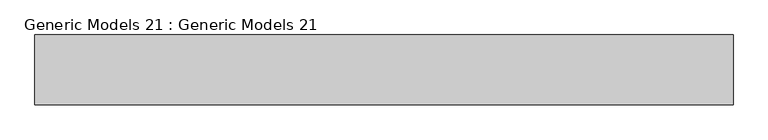
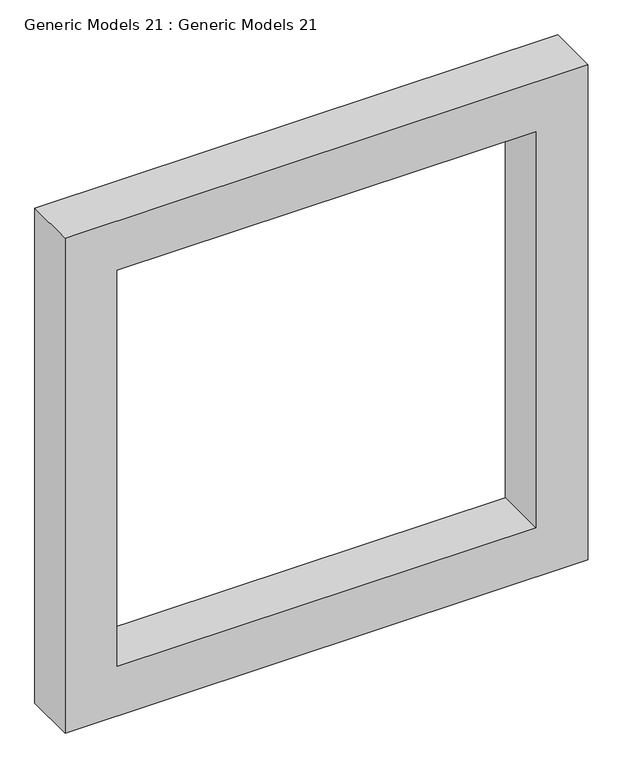
"""IFC4 building model written with IfcOpenShell, lengths in millimetres: proxy geometry, Generic Models 21 : Generic Models 21."""

from ifc_helpers import new_model, si_unit, frame, origin, place, context, project, spatial, polyline, outline, extrude, source, transform, mapped, element, save


def generic_models_21_generic_models_21_07dc1754(model_context):
    return source(origin(), model_context, "Body", "SweptSolid", [
        extrude(outline(polyline([(11820.4, 5704.5916602), (11820.4, 4180.5916602), (10296.4, 4180.5916602), (10296.4, 5704.5916602), (11820.4, 5704.5916602)]), holes=[polyline([(11668.0, 5552.1916602), (10448.8, 5552.1916602), (10448.8, 4332.9916602), (11668.0, 4332.9916602), (11668.0, 5552.1916602)])]), frame((0.0, -11268.8679047, 0.0), z_axis=(0.0, 1.0, 0.0), x_axis=(0.0, 0.0, 1.0)), (0.0, 0.0, 1.0), 152.4),
    ])


if __name__ == "__main__":
    model = new_model("IFC4")
    model_context = context("Model", 3, world=origin())
    ifc_project = project(units=[si_unit("LENGTHUNIT", "METRE", prefix="MILLI")], contexts=[model_context])
    site = spatial("IfcSite", under=ifc_project)
    building = spatial("IfcBuilding", under=site)
    placement = place(None, origin())
    generic_models_21_generic_models_21_shape = generic_models_21_generic_models_21_07dc1754(model_context)
    element("IfcBuildingElementProxy", 1, Name="Generic Models 21 : Generic Models 21", ObjectType="Generic Models 21 : Generic Models 21", at=placement, inside=building, context=model_context, shape_type="MappedRepresentation", body=[
        mapped(generic_models_21_generic_models_21_shape, transform((0.0, 0.0, 0.0), x_axis=(1.0, 0.0, 0.0), y_axis=(0.0, 1.0, 0.0), z_axis=(0.0, 0.0, 1.0))),
    ])
    save(model, "model.ifc")

# Revit data of these elements
# Element 1 (IfcBuildingElementProxy, "Generic Models 21 : Generic Models 21")
#   Materials on its faces: "TEAK BROWN COLOUR"
# Materials
#   "TEAK BROWN COLOUR": class "Generic", colour RGB 120 120 120, transparency 0, Cost = 0
